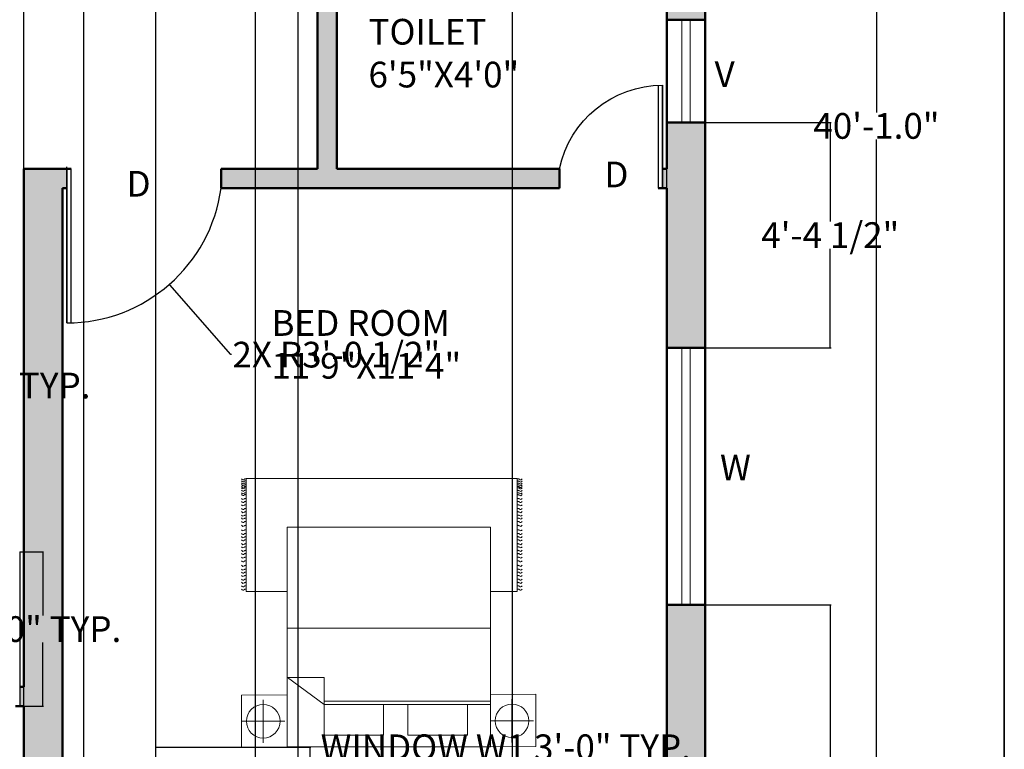
# Model space of a CAD drawing. Units: inches. Extents: x 125920 to 126336, y 366134 to 366735.
# Tile 3 of 6: x 126106 to 126336, y 366303 to 366473. Entities that reach past the tile are written whole.
import ezdxf

# ---------------------------------------------------------------- set-up
doc = ezdxf.new("R2010")
doc.units = ezdxf.units.IN
doc.header["$MEASUREMENT"] = 0
for name, color, linetype, lineweight in [('A-ANNO-DIMS', 2, 'Continuous', 18), ('A-ANNO-TEXT', 7, 'Continuous', 18), ('A-ANNO-TTLB', 7, 'Continuous', 35), ('A-AREA-IDEN', 7, 'Continuous', 25), ('A-DOOR', 3, 'Continuous', 25), ('A-FURN', 8, 'Continuous', 18), ('A-GLAZ', 4, 'Continuous', 18), ('A-WALL', 7, 'Continuous', 50)]:
    doc.layers.add(name, color=color, linetype=linetype, lineweight=lineweight)
doc.layers.add('A-WALL-PATT', color=18, linetype='Continuous', lineweight=13, true_color=0x000000)
doc.styles.get("Standard").update_dxf_attribs({"font": 'arial.ttf'})
doc.dimstyles.get("Standard").update_dxf_attribs({"dimtxt": 6, "dimasz": 0.18, "dimexe": 0.18, "dimexo": 0.0625, "dimgap": 0.09, "dimtad": 0, "dimtih": 1, "dimtoh": 1, "dimdec": 1, "dimzin": 0, "dimdsep": 46, "dimlunit": 3, "dimtxsty": 'Standard', "dimcen": 0.09, "dimadec": 0, "dimazin": 0, "dimtfac": 1, "dimtdec": 1, "dimtofl": 0, "dimtmove": 0, "dimatfit": 3, "dimfxl": 1, "dimtolj": 1, "dimtzin": 0, "dimarcsym": 0})

# ---------------------------------------------------------------- blocks, each defined once
blk = doc.blocks.new('*D4')
at = {"layer": 'A-ANNO-DIMS', "color": 0, "lineweight": -2, "transparency": 16777216}
for p, q in [((126266.54, 366688.79), (126306.57, 366688.79)), ((126306.39, 366688.61), (126306.39, 366451.45)), ((126306.39, 366207.97), (126306.39, 366445.14)), ((126266.54, 366207.79), (126306.57, 366207.79))]:
    blk.add_line(p, q, dxfattribs=at)
at = {"layer": 'A-ANNO-DIMS', "color": 0, "transparency": 16777216}
for points in [[(126306.36, 366688.61), (126306.42, 366688.61), (126306.39, 366688.79)], [(126306.36, 366207.97), (126306.42, 366207.97), (126306.39, 366207.79)]]:
    blk.add_solid(points, dxfattribs=at)
at = {"layer": 'Defpoints', "color": 0, "transparency": 16777216}
for p in [(126266.47, 366688.79), (126266.47, 366207.79), (126306.39, 366207.79)]:
    blk.add_point(p, dxfattribs=at)
at = {"layer": 'A-ANNO-DIMS', "color": 0, "transparency": 16777216, "insert": (126306.39, 366448.29), "char_height": 6, "attachment_point": 5}
blk.add_mtext('\\A1;40\'-1.0"', dxfattribs=at)
blk = doc.blocks.new('BED-DOUBLE-WITH-NIGHTSTANDS')
for p, q in [((5.6, 61.62), (5.6, 51.56)), ((63.65, 61.72), (63.65, 51.66)), ((10.63, 56.59), (0.57, 56.59)), ((68.68, 56.69), (58.62, 56.69)), ((49.39, 52.82), (10.63, 52.82)), ((49.44, 52), (10.63, 52)), ((49.39, 52.82), (58, 46.47)), ((49.44, 52.82), (49.44, 46.47)), ((49.44, 46.47), (58, 46.47)), ((58.05, 34.96), (10.63, 34.96)), ((4.36, 0), (4.36, 26.37)), ((4.36, 26.37), (10.65, 26.37)), ((58.05, 26.37), (67.59, 26.37)), ((67.59, 26.37), (67.59, 0)), ((67.59, 0), (4.36, 0))]:
    blk.add_line(p, q)
for points in [[(0, 50.39), (10.63, 50.5), (10.63, 62.68), (0, 62.58)], [(58.05, 62.68), (58.05, 11.37), (10.63, 11.37), (10.63, 62.68)], [(58.05, 50.5), (68.68, 50.6), (68.68, 62.78), (58.05, 62.68)], [(29.88, 59.98), (29.88, 52.82), (15.98, 52.82), (15.98, 59.98)], [(49.44, 59.98), (49.44, 52.82), (35.55, 52.82), (35.55, 59.98)]]:
    blk.add_lwpolyline(points, close=True)
for centre in [(5.6, 56.59), (63.65, 56.69)]:
    blk.add_circle(centre, 3.92)
for points, knots in [([(3.23, 25.84), (3.32, 25.96), (3.52, 26.2), (3.86, 25.96), (4.14, 25.78), (4.29, 25.89), (4.36, 25.94)], [0, 0, 0, 0, 0.400747, 0.791423, 1.067667, 1.29709, 1.29709, 1.29709, 1.29709]), ([(3.23, 25.06), (3.32, 25.18), (3.52, 25.42), (3.86, 25.18), (4.14, 25.01), (4.29, 25.11), (4.36, 25.16)], [0, 0, 0, 0, 0.400747, 0.791423, 1.067667, 1.29709, 1.29709, 1.29709, 1.29709]), ([(68.71, 25.84), (68.61, 25.96), (68.42, 26.2), (68.08, 25.96), (67.8, 25.78), (67.65, 25.89), (67.58, 25.94)], [0, 0, 0, 0, 0.400747, 0.791423, 1.067667, 1.29709, 1.29709, 1.29709, 1.29709]), ([(68.71, 25.06), (68.61, 25.18), (68.42, 25.42), (68.08, 25.18), (67.8, 25.01), (67.65, 25.11), (67.58, 25.16)], [0, 0, 0, 0, 0.400747, 0.791423, 1.067667, 1.29709, 1.29709, 1.29709, 1.29709]), ([(3.23, 24.24), (3.32, 24.36), (3.52, 24.6), (3.86, 24.36), (4.14, 24.19), (4.29, 24.3), (4.36, 24.34)], [0, 0, 0, 0, 0.400747, 0.791423, 1.067667, 1.29709, 1.29709, 1.29709, 1.29709]), ([(3.23, 23.51), (3.32, 23.63), (3.52, 23.87), (3.86, 23.63), (4.14, 23.46), (4.29, 23.57), (4.36, 23.62)], [0, 0, 0, 0, 0.400747, 0.791423, 1.067667, 1.29709, 1.29709, 1.29709, 1.29709]), ([(68.71, 24.24), (68.61, 24.36), (68.42, 24.6), (68.08, 24.36), (67.8, 24.19), (67.65, 24.3), (67.58, 24.34)], [0, 0, 0, 0, 0.400747, 0.791423, 1.067667, 1.29709, 1.29709, 1.29709, 1.29709]), ([(68.71, 23.51), (68.61, 23.63), (68.42, 23.87), (68.08, 23.63), (67.8, 23.46), (67.65, 23.57), (67.58, 23.62)], [0, 0, 0, 0, 0.400747, 0.791423, 1.067667, 1.29709, 1.29709, 1.29709, 1.29709]), ([(3.23, 22.63), (3.32, 22.75), (3.52, 22.99), (3.86, 22.75), (4.14, 22.58), (4.29, 22.69), (4.36, 22.73)], [0, 0, 0, 0, 0.400747, 0.791423, 1.067667, 1.29709, 1.29709, 1.29709, 1.29709]), ([(3.23, 21.88), (3.32, 22), (3.52, 22.24), (3.86, 22), (4.14, 21.83), (4.29, 21.93), (4.36, 21.98)], [0, 0, 0, 0, 0.400747, 0.791423, 1.067667, 1.29709, 1.29709, 1.29709, 1.29709]), ([(3.23, 21.15), (3.32, 21.27), (3.52, 21.51), (3.86, 21.27), (4.14, 21.1), (4.29, 21.21), (4.36, 21.25)], [0, 0, 0, 0, 0.400747, 0.791423, 1.067667, 1.29709, 1.29709, 1.29709, 1.29709]), ([(68.71, 22.63), (68.61, 22.75), (68.42, 22.99), (68.08, 22.75), (67.8, 22.58), (67.65, 22.69), (67.58, 22.73)], [0, 0, 0, 0, 0.400747, 0.791423, 1.067667, 1.29709, 1.29709, 1.29709, 1.29709]), ([(68.71, 21.88), (68.61, 22), (68.42, 22.24), (68.08, 22), (67.8, 21.83), (67.65, 21.93), (67.58, 21.98)], [0, 0, 0, 0, 0.400747, 0.791423, 1.067667, 1.29709, 1.29709, 1.29709, 1.29709]), ([(68.71, 21.15), (68.61, 21.27), (68.42, 21.51), (68.08, 21.27), (67.8, 21.1), (67.65, 21.21), (67.58, 21.25)], [0, 0, 0, 0, 0.400747, 0.791423, 1.067667, 1.29709, 1.29709, 1.29709, 1.29709]), ([(3.23, 20.27), (3.32, 20.39), (3.52, 20.63), (3.86, 20.39), (4.14, 20.22), (4.29, 20.32), (4.36, 20.37)], [0, 0, 0, 0, 0.400747, 0.791423, 1.067667, 1.29709, 1.29709, 1.29709, 1.29709]), ([(3.23, 19.23), (3.32, 19.35), (3.52, 19.59), (3.86, 19.35), (4.14, 19.18), (4.29, 19.29), (4.36, 19.33)], [0, 0, 0, 0, 0.400747, 0.791423, 1.067667, 1.29709, 1.29709, 1.29709, 1.29709]), ([(3.23, 18.35), (3.32, 18.47), (3.52, 18.71), (3.86, 18.47), (4.14, 18.3), (4.29, 18.4), (4.36, 18.45)], [0, 0, 0, 0, 0.400747, 0.791423, 1.067667, 1.29709, 1.29709, 1.29709, 1.29709]), ([(68.71, 20.27), (68.61, 20.39), (68.42, 20.63), (68.08, 20.39), (67.8, 20.22), (67.65, 20.32), (67.58, 20.37)], [0, 0, 0, 0, 0.400747, 0.791423, 1.067667, 1.29709, 1.29709, 1.29709, 1.29709]), ([(68.71, 19.23), (68.61, 19.35), (68.42, 19.59), (68.08, 19.35), (67.8, 19.18), (67.65, 19.29), (67.58, 19.33)], [0, 0, 0, 0, 0.400747, 0.791423, 1.067667, 1.29709, 1.29709, 1.29709, 1.29709]), ([(68.71, 18.35), (68.61, 18.47), (68.42, 18.71), (68.08, 18.47), (67.8, 18.3), (67.65, 18.4), (67.58, 18.45)], [0, 0, 0, 0, 0.400747, 0.791423, 1.067667, 1.29709, 1.29709, 1.29709, 1.29709]), ([(3.23, 17.53), (3.32, 17.65), (3.52, 17.89), (3.86, 17.65), (4.14, 17.48), (4.29, 17.59), (4.36, 17.64)], [0, 0, 0, 0, 0.400747, 0.791423, 1.067667, 1.29709, 1.29709, 1.29709, 1.29709]), ([(3.23, 16.76), (3.32, 16.88), (3.52, 17.12), (3.86, 16.88), (4.14, 16.7), (4.29, 16.81), (4.36, 16.86)], [0, 0, 0, 0, 0.400747, 0.791423, 1.067667, 1.29709, 1.29709, 1.29709, 1.29709]), ([(3.23, 15.94), (3.32, 16.06), (3.52, 16.3), (3.86, 16.06), (4.14, 15.89), (4.29, 16), (4.36, 16.04)], [0, 0, 0, 0, 0.400747, 0.791423, 1.067667, 1.29709, 1.29709, 1.29709, 1.29709]), ([(68.71, 17.53), (68.61, 17.65), (68.42, 17.89), (68.08, 17.65), (67.8, 17.48), (67.65, 17.59), (67.58, 17.64)], [0, 0, 0, 0, 0.400747, 0.791423, 1.067667, 1.29709, 1.29709, 1.29709, 1.29709]), ([(68.71, 16.76), (68.61, 16.88), (68.42, 17.12), (68.08, 16.88), (67.8, 16.7), (67.65, 16.81), (67.58, 16.86)], [0, 0, 0, 0, 0.400747, 0.791423, 1.067667, 1.29709, 1.29709, 1.29709, 1.29709]), ([(68.71, 15.94), (68.61, 16.06), (68.42, 16.3), (68.08, 16.06), (67.8, 15.89), (67.65, 16), (67.58, 16.04)], [0, 0, 0, 0, 0.400747, 0.791423, 1.067667, 1.29709, 1.29709, 1.29709, 1.29709]), ([(3.23, 15.21), (3.32, 15.33), (3.52, 15.57), (3.86, 15.33), (4.14, 15.16), (4.29, 15.27), (4.36, 15.32)], [0, 0, 0, 0, 0.400747, 0.791423, 1.067667, 1.29709, 1.29709, 1.29709, 1.29709]), ([(3.23, 14.33), (3.32, 14.45), (3.52, 14.69), (3.86, 14.45), (4.14, 14.28), (4.29, 14.38), (4.36, 14.43)], [0, 0, 0, 0, 0.400747, 0.791423, 1.067667, 1.29709, 1.29709, 1.29709, 1.29709]), ([(3.23, 13.58), (3.32, 13.7), (3.52, 13.94), (3.86, 13.7), (4.14, 13.53), (4.29, 13.63), (4.36, 13.68)], [0, 0, 0, 0, 0.400747, 0.791423, 1.067667, 1.29709, 1.29709, 1.29709, 1.29709]), ([(68.71, 15.21), (68.61, 15.33), (68.42, 15.57), (68.08, 15.33), (67.8, 15.16), (67.65, 15.27), (67.58, 15.32)], [0, 0, 0, 0, 0.400747, 0.791423, 1.067667, 1.29709, 1.29709, 1.29709, 1.29709]), ([(68.71, 14.33), (68.61, 14.45), (68.42, 14.69), (68.08, 14.45), (67.8, 14.28), (67.65, 14.38), (67.58, 14.43)], [0, 0, 0, 0, 0.400747, 0.791423, 1.067667, 1.29709, 1.29709, 1.29709, 1.29709]), ([(68.71, 13.58), (68.61, 13.7), (68.42, 13.94), (68.08, 13.7), (67.8, 13.53), (67.65, 13.63), (67.58, 13.68)], [0, 0, 0, 0, 0.400747, 0.791423, 1.067667, 1.29709, 1.29709, 1.29709, 1.29709]), ([(3.23, 12.85), (3.32, 12.97), (3.52, 13.21), (3.86, 12.97), (4.14, 12.8), (4.29, 12.9), (4.36, 12.95)], [0, 0, 0, 0, 0.400747, 0.791423, 1.067667, 1.29709, 1.29709, 1.29709, 1.29709]), ([(3.23, 11.97), (3.32, 12.09), (3.52, 12.33), (3.86, 12.09), (4.14, 11.92), (4.29, 12.02), (4.36, 12.07)], [0, 0, 0, 0, 0.400747, 0.791423, 1.067667, 1.29709, 1.29709, 1.29709, 1.29709]), ([(68.71, 12.85), (68.61, 12.97), (68.42, 13.21), (68.08, 12.97), (67.8, 12.8), (67.65, 12.9), (67.58, 12.95)], [0, 0, 0, 0, 0.400747, 0.791423, 1.067667, 1.29709, 1.29709, 1.29709, 1.29709]), ([(68.71, 11.97), (68.61, 12.09), (68.42, 12.33), (68.08, 12.09), (67.8, 11.92), (67.65, 12.02), (67.58, 12.07)], [0, 0, 0, 0, 0.400747, 0.791423, 1.067667, 1.29709, 1.29709, 1.29709, 1.29709]), ([(3.23, 10.93), (3.32, 11.05), (3.52, 11.29), (3.86, 11.05), (4.14, 10.88), (4.29, 10.99), (4.36, 11.03)], [0, 0, 0, 0, 0.400747, 0.791423, 1.067667, 1.29709, 1.29709, 1.29709, 1.29709]), ([(3.23, 10.05), (3.32, 10.17), (3.52, 10.41), (3.86, 10.17), (4.14, 10), (4.29, 10.1), (4.36, 10.15)], [0, 0, 0, 0, 0.400747, 0.791423, 1.067667, 1.29709, 1.29709, 1.29709, 1.29709]), ([(3.23, 9.23), (3.32, 9.35), (3.52, 9.59), (3.86, 9.35), (4.14, 9.18), (4.29, 9.29), (4.36, 9.34)], [0, 0, 0, 0, 0.400747, 0.791423, 1.067667, 1.29709, 1.29709, 1.29709, 1.29709]), ([(68.71, 10.93), (68.61, 11.05), (68.42, 11.29), (68.08, 11.05), (67.8, 10.88), (67.65, 10.99), (67.58, 11.03)], [0, 0, 0, 0, 0.400747, 0.791423, 1.067667, 1.29709, 1.29709, 1.29709, 1.29709]), ([(68.71, 10.05), (68.61, 10.17), (68.42, 10.41), (68.08, 10.17), (67.8, 10), (67.65, 10.1), (67.58, 10.15)], [0, 0, 0, 0, 0.400747, 0.791423, 1.067667, 1.29709, 1.29709, 1.29709, 1.29709]), ([(68.71, 9.23), (68.61, 9.35), (68.42, 9.59), (68.08, 9.35), (67.8, 9.18), (67.65, 9.29), (67.58, 9.34)], [0, 0, 0, 0, 0.400747, 0.791423, 1.067667, 1.29709, 1.29709, 1.29709, 1.29709]), ([(3.23, 8.54), (3.32, 8.66), (3.52, 8.9), (3.86, 8.66), (4.14, 8.49), (4.29, 8.6), (4.36, 8.65)], [0, 0, 0, 0, 0.400747, 0.791423, 1.067667, 1.29709, 1.29709, 1.29709, 1.29709]), ([(3.23, 7.73), (3.32, 7.85), (3.52, 8.09), (3.86, 7.85), (4.14, 7.68), (4.29, 7.78), (4.36, 7.83)], [0, 0, 0, 0, 0.400747, 0.791423, 1.067667, 1.29709, 1.29709, 1.29709, 1.29709]), ([(3.23, 7), (3.32, 7.12), (3.52, 7.36), (3.86, 7.12), (4.14, 6.95), (4.29, 7.05), (4.36, 7.1)], [0, 0, 0, 0, 0.400747, 0.791423, 1.067667, 1.29709, 1.29709, 1.29709, 1.29709]), ([(68.71, 8.54), (68.61, 8.66), (68.42, 8.9), (68.08, 8.66), (67.8, 8.49), (67.65, 8.6), (67.58, 8.65)], [0, 0, 0, 0, 0.400747, 0.791423, 1.067667, 1.29709, 1.29709, 1.29709, 1.29709]), ([(68.71, 7.73), (68.61, 7.85), (68.42, 8.09), (68.08, 7.85), (67.8, 7.68), (67.65, 7.78), (67.58, 7.83)], [0, 0, 0, 0, 0.400747, 0.791423, 1.067667, 1.29709, 1.29709, 1.29709, 1.29709]), ([(68.71, 7), (68.61, 7.12), (68.42, 7.36), (68.08, 7.12), (67.8, 6.95), (67.65, 7.05), (67.58, 7.1)], [0, 0, 0, 0, 0.400747, 0.791423, 1.067667, 1.29709, 1.29709, 1.29709, 1.29709]), ([(3.23, 6.12), (3.32, 6.24), (3.52, 6.48), (3.86, 6.24), (4.14, 6.07), (4.29, 6.17), (4.36, 6.22)], [0, 0, 0, 0, 0.400747, 0.791423, 1.067667, 1.29709, 1.29709, 1.29709, 1.29709]), ([(3.23, 5.36), (3.32, 5.49), (3.52, 5.73), (3.86, 5.49), (4.14, 5.31), (4.29, 5.42), (4.36, 5.47)], [0, 0, 0, 0, 0.400747, 0.791423, 1.067667, 1.29709, 1.29709, 1.29709, 1.29709]), ([(3.23, 4.64), (3.32, 4.76), (3.52, 5), (3.86, 4.76), (4.14, 4.59), (4.29, 4.69), (4.36, 4.74)], [0, 0, 0, 0, 0.400747, 0.791423, 1.067667, 1.29709, 1.29709, 1.29709, 1.29709]), ([(68.71, 6.12), (68.61, 6.24), (68.42, 6.48), (68.08, 6.24), (67.8, 6.07), (67.65, 6.17), (67.58, 6.22)], [0, 0, 0, 0, 0.400747, 0.791423, 1.067667, 1.29709, 1.29709, 1.29709, 1.29709]), ([(68.71, 5.36), (68.61, 5.49), (68.42, 5.73), (68.08, 5.49), (67.8, 5.31), (67.65, 5.42), (67.58, 5.47)], [0, 0, 0, 0, 0.400747, 0.791423, 1.067667, 1.29709, 1.29709, 1.29709, 1.29709]), ([(68.71, 4.64), (68.61, 4.76), (68.42, 5), (68.08, 4.76), (67.8, 4.59), (67.66, 4.69), (67.59, 4.73)], [0, 0, 0, 0, 0.400747, 0.791423, 1.067667, 1.283686, 1.283686, 1.283686, 1.283686]), ([(3.23, 3.75), (3.32, 3.88), (3.52, 4.12), (3.86, 3.88), (4.14, 3.7), (4.29, 3.81), (4.36, 3.86)], [0, 0, 0, 0, 0.400747, 0.791423, 1.067667, 1.29709, 1.29709, 1.29709, 1.29709]), ([(3.23, 3.33), (3.32, 3.45), (3.52, 3.7), (3.86, 3.44), (4.14, 3.27), (4.29, 3.38), (4.36, 3.43)], [0, 0, 0, 0, 0.407265, 0.802015, 1.07826, 1.307683, 1.307683, 1.307683, 1.307683]), ([(3.23, 2.76), (3.32, 2.88), (3.52, 3.12), (3.86, 2.88), (4.14, 2.71), (4.29, 2.81), (4.36, 2.86)], [0, 0, 0, 0, 0.400747, 0.791423, 1.067667, 1.29709, 1.29709, 1.29709, 1.29709]), ([(3.23, 2.18), (3.32, 2.31), (3.52, 2.55), (3.86, 2.31), (4.14, 2.13), (4.29, 2.24), (4.36, 2.29)], [0, 0, 0, 0, 0.400747, 0.791423, 1.067667, 1.29709, 1.29709, 1.29709, 1.29709]), ([(68.71, 3.75), (68.61, 3.88), (68.42, 4.11), (68.08, 3.88), (67.8, 3.7), (67.66, 3.81), (67.59, 3.85)], [0, 0, 0, 0, 0.400747, 0.791423, 1.067667, 1.283686, 1.283686, 1.283686, 1.283686]), ([(68.71, 3.33), (68.61, 3.45), (68.42, 3.69), (68.08, 3.45), (67.8, 3.27), (67.66, 3.38), (67.59, 3.42)], [0, 0, 0, 0, 0.402903, 0.794912, 1.071156, 1.287177, 1.287177, 1.287177, 1.287177]), ([(68.71, 2.73), (68.61, 2.85), (68.42, 3.09), (68.08, 2.85), (67.8, 2.68), (67.66, 2.78), (67.59, 2.82)], [0, 0, 0, 0, 0.400747, 0.791423, 1.067667, 1.283686, 1.283686, 1.283686, 1.283686]), ([(68.71, 2.16), (68.61, 2.28), (68.42, 2.52), (68.08, 2.28), (67.8, 2.11), (67.66, 2.21), (67.59, 2.25)], [0, 0, 0, 0, 0.400747, 0.791423, 1.067667, 1.283686, 1.283686, 1.283686, 1.283686]), ([(3.23, 1.88), (3.32, 2), (3.52, 2.24), (3.86, 2), (4.14, 1.82), (4.29, 1.93), (4.36, 1.98)], [0, 0, 0, 0, 0.400747, 0.791423, 1.067667, 1.29709, 1.29709, 1.29709, 1.29709]), ([(3.23, 1.46), (3.32, 1.58), (3.52, 1.82), (3.86, 1.58), (4.14, 1.41), (4.29, 1.51), (4.36, 1.56)], [0, 0, 0, 0, 0.400747, 0.791423, 1.067667, 1.29709, 1.29709, 1.29709, 1.29709]), ([(3.23, 1.06), (3.32, 1.18), (3.52, 1.42), (3.86, 1.18), (4.14, 1.01), (4.29, 1.11), (4.36, 1.16)], [0, 0, 0, 0, 0.400747, 0.791423, 1.067667, 1.29709, 1.29709, 1.29709, 1.29709]), ([(3.23, 0.57), (3.32, 0.7), (3.52, 0.94), (3.86, 0.7), (4.14, 0.52), (4.29, 0.63), (4.36, 0.68)], [0, 0, 0, 0, 0.400747, 0.791423, 1.067667, 1.29709, 1.29709, 1.29709, 1.29709]), ([(3.23, 0.07), (3.32, 0.19), (3.52, 0.43), (3.86, 0.19), (4.14, 0.02), (4.29, 0.13), (4.36, 0.18)], [0, 0, 0, 0, 0.400747, 0.791423, 1.067667, 1.29709, 1.29709, 1.29709, 1.29709]), ([(68.71, 1.43), (68.61, 1.55), (68.42, 1.79), (68.08, 1.55), (67.8, 1.38), (67.65, 1.48), (67.58, 1.53)], [0, 0, 0, 0, 0.400747, 0.791423, 1.067667, 1.29709, 1.29709, 1.29709, 1.29709]), ([(68.71, 1.03), (68.61, 1.15), (68.42, 1.39), (68.08, 1.15), (67.8, 0.98), (67.65, 1.09), (67.58, 1.13)], [0, 0, 0, 0, 0.400747, 0.791423, 1.067667, 1.29709, 1.29709, 1.29709, 1.29709]), ([(68.71, 0.55), (68.61, 0.67), (68.42, 0.91), (68.08, 0.67), (67.8, 0.49), (67.65, 0.6), (67.58, 0.65)], [0, 0, 0, 0, 0.400747, 0.791423, 1.067667, 1.29709, 1.29709, 1.29709, 1.29709]), ([(68.71, 0.07), (68.61, 0.19), (68.42, 0.43), (68.08, 0.19), (67.8, 0.02), (67.65, 0.13), (67.58, 0.18)], [0, 0, 0, 0, 0.400747, 0.791423, 1.067667, 1.29709, 1.29709, 1.29709, 1.29709]), ([(68.71, 1.85), (68.61, 1.97), (68.42, 2.21), (68.08, 1.97), (67.8, 1.8), (67.66, 1.9), (67.59, 1.94)], [0, 0, 0, 0, 0.400747, 0.791423, 1.067667, 1.283686, 1.283686, 1.283686, 1.283686])]:
    blk.add_open_spline(points, degree=3, knots=knots)
blk = doc.blocks.new('WIN-60')
for p, q in [((0, 0), (0, 60)), ((3.5, 0), (3.5, 60)), ((5.5, 60), (5.5, 0)), ((9, 60), (9, 0))]:
    blk.add_line(p, q)
blk = doc.blocks.new('VENT-24')
for p, q in [((0, 0), (0, 24)), ((3.5, 0), (3.5, 24)), ((5.5, 24), (5.5, 0)), ((9, 24), (9, 0))]:
    blk.add_line(p, q)
blk = doc.blocks.new('DOOR-36-WALL-4_5')
for p, q in [((0, 36), (0, 0)), ((0, 36), (1, 36)), ((1, 0), (1, 36))]:
    blk.add_line(p, q)
blk.add_arc((0, 36.32), 36.32, 270, 352.3719)
blk = doc.blocks.new('DOOR-24-WALL-4_5')
for p, q in [((0, 1), (24, 1)), ((24, 0), (24, 1)), ((24, 0), (0, 0))]:
    blk.add_line(p, q)
blk.add_arc((24.52, 0), 24.52, 101.8123, 180)
blk = doc.blocks.new('*D15')
at = {"layer": 'A-ANNO-DIMS', "color": 0, "lineweight": -2, "transparency": 16777216}
for p, q in [((126138.23, 366297.86), (126138.23, 366303.37)), ((126138.41, 366303.19), (126174.05, 366303.19)), ((126174.23, 366297.86), (126174.23, 366303.37)), ((126174.23, 366303.19), (126174.41, 366303.19))]:
    blk.add_line(p, q, dxfattribs=at)
at = {"layer": 'A-ANNO-DIMS', "color": 0, "transparency": 16777216}
for points in [[(126138.41, 366303.22), (126138.41, 366303.16), (126138.23, 366303.19)], [(126174.05, 366303.22), (126174.05, 366303.16), (126174.23, 366303.19)]]:
    blk.add_solid(points, dxfattribs=at)
at = {"layer": 'Defpoints', "color": 0, "transparency": 16777216}
for p in [(126174.23, 366303.19), (126138.23, 366297.79), (126174.23, 366297.79)]:
    blk.add_point(p, dxfattribs=at)
at = {"layer": 'A-ANNO-DIMS', "color": 0, "transparency": 16777216, "insert": (126219.91, 366303.19), "char_height": 6, "attachment_point": 5}
blk.add_mtext('\\A1;WINDOW W1 3\'-0" TYP.', dxfattribs=at)
blk = doc.blocks.new('*D21')
at = {"layer": 'A-ANNO-DIMS', "color": 0, "lineweight": -2, "transparency": 16777216}
for p, q in [((126007.38, 366379.47), (126007.38, 366387.84)), ((126007.56, 366387.66), (126062.24, 366387.66)), ((126062.42, 366379.47), (126062.42, 366387.84)), ((126062.42, 366387.66), (126062.6, 366387.66))]:
    blk.add_line(p, q, dxfattribs=at)
at = {"layer": 'A-ANNO-DIMS', "color": 0, "transparency": 16777216}
for points in [[(126007.56, 366387.69), (126007.56, 366387.63), (126007.38, 366387.66)], [(126062.24, 366387.69), (126062.24, 366387.63), (126062.42, 366387.66)]]:
    blk.add_solid(points, dxfattribs=at)
at = {"layer": 'Defpoints', "color": 0, "transparency": 16777216}
for p in [(126062.42, 366387.66), (126007.38, 366379.4), (126062.42, 366379.4)]:
    blk.add_point(p, dxfattribs=at)
at = {"layer": 'A-ANNO-DIMS', "color": 0, "transparency": 16777216, "insert": (126093.54, 366387.66), "char_height": 6, "attachment_point": 5}
blk.add_mtext('\\A1;SOFA 4\'-7" TYP.', dxfattribs=at)
blk = doc.blocks.new('*D24')
at = {"layer": 'A-ANNO-DIMS', "color": 0, "lineweight": -2, "transparency": 16777216}
for p, q in [((126106.54, 366348.79), (126112.05, 366348.79)), ((126111.87, 366348.61), (126111.87, 366333.95)), ((126111.87, 366312.97), (126111.87, 366327.64)), ((126106.54, 366312.79), (126112.05, 366312.79))]:
    blk.add_line(p, q, dxfattribs=at)
at = {"layer": 'A-ANNO-DIMS', "color": 0, "transparency": 16777216}
for points in [[(126111.84, 366348.61), (126111.9, 366348.61), (126111.87, 366348.79)], [(126111.84, 366312.97), (126111.9, 366312.97), (126111.87, 366312.79)]]:
    blk.add_solid(points, dxfattribs=at)
at = {"layer": 'Defpoints', "color": 0, "transparency": 16777216}
for p in [(126106.47, 366348.79), (126106.47, 366312.79), (126111.87, 366312.79)]:
    blk.add_point(p, dxfattribs=at)
at = {"layer": 'A-ANNO-DIMS', "color": 0, "transparency": 16777216, "insert": (126111.87, 366330.79), "char_height": 6, "attachment_point": 5}
blk.add_mtext('\\A1;3\'-0" TYP.', dxfattribs=at)
blk = doc.blocks.new('*D32')
at = {"layer": 'A-ANNO-DIMS', "color": 0, "lineweight": -2, "transparency": 16777216}
for p, q in [((126266.54, 366336.48), (126295.8, 366336.48)), ((126295.62, 366336.3), (126295.62, 366275.33)), ((126295.62, 366207.97), (126295.62, 366268.94)), ((126266.54, 366207.79), (126295.8, 366207.79))]:
    blk.add_line(p, q, dxfattribs=at)
at = {"layer": 'A-ANNO-DIMS', "color": 0, "transparency": 16777216}
for points in [[(126295.59, 366336.3), (126295.65, 366336.3), (126295.62, 366336.48)], [(126295.59, 366207.97), (126295.65, 366207.97), (126295.62, 366207.79)]]:
    blk.add_solid(points, dxfattribs=at)
at = {"layer": 'Defpoints', "color": 0, "transparency": 16777216}
for p in [(126266.47, 366336.48), (126295.62, 366336.48), (126266.47, 366207.79)]:
    blk.add_point(p, dxfattribs=at)
at = {"layer": 'A-ANNO-DIMS', "color": 0, "transparency": 16777216, "insert": (126295.62, 366272.14), "char_height": 6, "attachment_point": 5}
blk.add_mtext('\\A1;10\'-8 1/2"', dxfattribs=at)
blk = doc.blocks.new('*D33')
at = {"layer": 'A-ANNO-DIMS', "color": 0, "lineweight": -2, "transparency": 16777216}
for p, q in [((126266.54, 366449.1), (126295.8, 366449.1)), ((126295.62, 366448.92), (126295.62, 366425.98)), ((126295.62, 366396.66), (126295.62, 366419.6)), ((126266.54, 366396.48), (126295.8, 366396.48))]:
    blk.add_line(p, q, dxfattribs=at)
at = {"layer": 'A-ANNO-DIMS', "color": 0, "transparency": 16777216}
for points in [[(126295.59, 366448.92), (126295.65, 366448.92), (126295.62, 366449.1)], [(126295.59, 366396.66), (126295.65, 366396.66), (126295.62, 366396.48)]]:
    blk.add_solid(points, dxfattribs=at)
at = {"layer": 'Defpoints', "color": 0, "transparency": 16777216}
for p in [(126266.47, 366449.1), (126295.62, 366449.1), (126266.47, 366396.48)]:
    blk.add_point(p, dxfattribs=at)
at = {"layer": 'A-ANNO-DIMS', "color": 0, "transparency": 16777216, "insert": (126295.62, 366422.79), "char_height": 6, "attachment_point": 5}
blk.add_mtext('\\A1;4\'-4 1/2"', dxfattribs=at)
blk = doc.blocks.new('*D40')
at = {"layer": 'A-ANNO-DIMS', "color": 0, "lineweight": -2, "transparency": 16777216}
for p, q in [((126107.47, 366288.86), (126107.47, 366718.12)), ((126107.65, 366717.94), (126114.73, 366717.94)), ((126138.05, 366717.94), (126130.97, 366717.94)), ((126138.23, 366288.86), (126138.23, 366718.12))]:
    blk.add_line(p, q, dxfattribs=at)
at = {"layer": 'A-ANNO-DIMS', "color": 0, "transparency": 16777216}
for points in [[(126107.65, 366717.97), (126107.65, 366717.91), (126107.47, 366717.94)], [(126138.05, 366717.97), (126138.05, 366717.91), (126138.23, 366717.94)]]:
    blk.add_solid(points, dxfattribs=at)
at = {"layer": 'Defpoints', "color": 0, "transparency": 16777216}
for p in [(126138.23, 366717.94), (126107.47, 366288.79), (126138.23, 366288.79)]:
    blk.add_point(p, dxfattribs=at)
at = {"layer": 'A-ANNO-DIMS', "color": 0, "transparency": 16777216, "insert": (126122.85, 366717.94), "char_height": 6, "attachment_point": 5}
blk.add_mtext('\\A1;2\'-7"', dxfattribs=at)
blk = doc.blocks.new('*D41')
at = {"layer": 'A-ANNO-DIMS', "color": 0, "lineweight": -2, "transparency": 16777216}
for p, q in [((126121.47, 366216.86), (126121.47, 366718.12)), ((126121.65, 366717.94), (126163.4, 366717.94)), ((126221.29, 366717.94), (126179.54, 366717.94)), ((126221.47, 366216.86), (126221.47, 366718.12))]:
    blk.add_line(p, q, dxfattribs=at)
at = {"layer": 'A-ANNO-DIMS', "color": 0, "transparency": 16777216}
for points in [[(126121.65, 366717.97), (126121.65, 366717.91), (126121.47, 366717.94)], [(126221.29, 366717.97), (126221.29, 366717.91), (126221.47, 366717.94)]]:
    blk.add_solid(points, dxfattribs=at)
at = {"layer": 'Defpoints', "color": 0, "transparency": 16777216}
for p in [(126221.47, 366717.94), (126121.47, 366216.79), (126221.47, 366216.79)]:
    blk.add_point(p, dxfattribs=at)
at = {"layer": 'A-ANNO-DIMS', "color": 0, "transparency": 16777216, "insert": (126171.47, 366717.94), "char_height": 6, "attachment_point": 5}
blk.add_mtext('\\A1;8\'-4"', dxfattribs=at)
blk = doc.blocks.new('*D43')
at = {"layer": 'A-ANNO-DIMS', "color": 0, "lineweight": -2, "transparency": 16777216}
for p, q in [((126221.47, 366216.86), (126221.47, 366718.12)), ((126221.65, 366717.94), (126231.41, 366717.94)), ((126257.29, 366717.94), (126247.54, 366717.94)), ((126257.47, 366216.86), (126257.47, 366718.12))]:
    blk.add_line(p, q, dxfattribs=at)
at = {"layer": 'A-ANNO-DIMS', "color": 0, "transparency": 16777216}
for points in [[(126221.65, 366717.97), (126221.65, 366717.91), (126221.47, 366717.94)], [(126257.29, 366717.97), (126257.29, 366717.91), (126257.47, 366717.94)]]:
    blk.add_solid(points, dxfattribs=at)
at = {"layer": 'Defpoints', "color": 0, "transparency": 16777216}
for p in [(126257.47, 366717.94), (126221.47, 366216.79), (126257.47, 366216.79)]:
    blk.add_point(p, dxfattribs=at)
at = {"layer": 'A-ANNO-DIMS', "color": 0, "transparency": 16777216, "insert": (126239.47, 366717.94), "char_height": 6, "attachment_point": 5}
blk.add_mtext('\\A1;3\'-0"', dxfattribs=at)
blk = doc.blocks.new('*D44')
at = {"layer": 'A-ANNO-DIMS', "color": 0, "lineweight": -2, "transparency": 16777216}
for p, q in [((126161.47, 366252.86), (126161.47, 366718.12)), ((126161.65, 366717.94), (126171.29, 366717.94)), ((126171.47, 366252.86), (126171.47, 366718.12)), ((126171.47, 366717.94), (126171.65, 366717.94))]:
    blk.add_line(p, q, dxfattribs=at)
at = {"layer": 'A-ANNO-DIMS', "color": 0, "transparency": 16777216}
for points in [[(126161.65, 366717.97), (126161.65, 366717.91), (126161.47, 366717.94)], [(126171.29, 366717.97), (126171.29, 366717.91), (126171.47, 366717.94)]]:
    blk.add_solid(points, dxfattribs=at)
at = {"layer": 'Defpoints', "color": 0, "transparency": 16777216}
for p in [(126171.47, 366717.94), (126161.47, 366252.79), (126171.47, 366252.79)]:
    blk.add_point(p, dxfattribs=at)
at = {"layer": 'A-ANNO-DIMS', "color": 0, "transparency": 16777216, "insert": (126182.05, 366717.94), "char_height": 6, "attachment_point": 5}
blk.add_mtext('\\A1;0\'-10"', dxfattribs=at)
blk = doc.blocks.new('*D49')
at = {"layer": 'A-ANNO-DIMS', "color": 0, "lineweight": -2, "transparency": 16777216}
for p, q in [((126117.38, 366438.62), (126117.56, 366438.62)), ((126117.47, 366438.53), (126117.47, 366438.71)), ((126155.74, 366394.88), (126141.51, 366411.15)), ((126155.92, 366394.88), (126155.74, 366394.88))]:
    blk.add_line(p, q, dxfattribs=at)
at = {"layer": 'A-ANNO-DIMS', "color": 0, "transparency": 16777216}
blk.add_solid([(126141.53, 366411.17), (126141.49, 366411.13), (126141.39, 366411.28)], dxfattribs=at)
at = {"layer": 'Defpoints', "color": 0, "transparency": 16777216}
for p in [(126117.47, 366438.62), (126141.39, 366411.28)]:
    blk.add_point(p, dxfattribs=at)
at = {"layer": 'A-ANNO-DIMS', "color": 0, "transparency": 16777216, "insert": (126180.35, 366394.88), "char_height": 6, "attachment_point": 5}
blk.add_mtext('\\A1;2X R3\'-0 1/2"', dxfattribs=at)

msp = doc.modelspace()

# ---------------------------------------------------------------- hatches: boundary and pattern name
at = {"layer": 'A-WALL-PATT'}
h = msp.add_hatch(color=256, dxfattribs=at)
h.dxf.hatch_style = 1
h.paths.add_polyline_path([(126266.47, 366688.79), (125966.47, 366688.79), (125966.47, 366649.55), (125975.47, 366649.55), (125975.47, 366679.79), (126107.47, 366679.79), (126107.47, 366547.79), (126106.47, 366547.79), (126106.47, 366538.79), (126107.47, 366538.79), (126117.47, 366538.79), (126117.47, 366547.79), (126116.47, 366547.79), (126116.47, 366679.79), (126257.47, 366679.79), (126257.47, 366648.33), (126266.47, 366648.33)])
h.paths.add_polyline_path([(126070.47, 366547.79), (125975.47, 366547.79), (125975.47, 366589.55), (125966.47, 366589.55), (125966.47, 366528.42), (125975.47, 366528.42), (125975.47, 366538.79), (126059.47, 366538.79), (126059.47, 366515.79), (126063.97, 366515.79), (126063.97, 366538.79), (126070.47, 366538.79)])
h.paths.add_polyline_path([(125975.47, 366486.29), (126063.97, 366486.29), (126063.97, 366491.79), (126059.47, 366491.79), (126059.47, 366490.79), (125975.47, 366490.79), (125975.47, 366504.42), (125966.47, 366504.42), (125966.47, 366437.07), (125975.47, 366437.07)])
h.paths.add_polyline_path([(125975.47, 366312.79), (126022.47, 366312.79), (126022.47, 366317.29), (125975.47, 366317.29), (125975.47, 366377.07), (125966.47, 366377.07), (125966.47, 366207.79), (125987.64, 366207.79), (125987.64, 366216.79), (125975.47, 366216.79)])
h.paths.add_polyline_path([(126063.97, 366216.79), (126063.97, 366312.79), (126070.47, 366312.79), (126070.47, 366317.29), (126058.47, 366317.29), (126058.47, 366312.79), (126059.47, 366312.79), (126059.47, 366216.79), (126047.64, 366216.79), (126047.64, 366207.79), (126063.97, 366207.79)])
h.paths.add_polyline_path([(126221.47, 366216.79), (126116.47, 366216.79), (126107.47, 366216.79), (126107.47, 366207.79), (126221.47, 366207.79)])
h.paths.add_polyline_path([(126266.47, 366336.48), (126257.47, 366336.48), (126257.47, 366297.79), (126174.23, 366297.79), (126174.23, 366288.79), (126257.47, 366288.79), (126257.47, 366207.79), (126266.47, 366207.79)])
h.paths.add_polyline_path([(126138.23, 366297.79), (126116.47, 366297.79), (126116.47, 366433.79), (126117.47, 366433.79), (126117.47, 366438.29), (126116.47, 366438.29), (126107.47, 366438.29), (126107.47, 366317.29), (126106.47, 366317.29), (126106.47, 366312.79), (126107.47, 366312.79), (126107.47, 366288.79), (126116.47, 366288.79), (126138.23, 366288.79)])
h.paths.add_polyline_path([(126266.47, 366449.1), (126257.47, 366449.1), (126257.47, 366438.29), (126256.47, 366438.29), (126256.47, 366433.79), (126257.47, 366433.79), (126257.47, 366396.48), (126266.47, 366396.48)])
h.paths.add_polyline_path([(126232.47, 366438.29), (126180.47, 366438.29), (126180.47, 366486.29), (126257.47, 366486.29), (126257.47, 366473.1), (126266.47, 366473.1), (126266.47, 366504.78), (126257.47, 366504.78), (126257.47, 366490.79), (126180.47, 366490.79), (126180.47, 366538.79), (126232.47, 366538.79), (126232.47, 366547.79), (126153.47, 366547.79), (126153.47, 366538.79), (126175.97, 366538.79), (126175.97, 366438.29), (126153.47, 366438.29), (126153.47, 366433.79), (126232.47, 366433.79)])
h.paths.add_polyline_path([(126266.47, 366588.33), (126257.47, 366588.33), (126257.47, 366547.79), (126256.47, 366547.79), (126256.47, 366538.79), (126257.47, 366538.79), (126257.47, 366528.78), (126266.47, 366528.78)])

# ---------------------------------------------------------------- linework, layer by layer
at = {"layer": 'A-ANNO-TTLB'}
msp.add_lwpolyline([(125932.73, 366735.48), (126336.24, 366735.48), (126336.24, 366133.52), (125932.73, 366133.52)], close=True, dxfattribs=at)
at = {"layer": 'A-DOOR'}
for p, q in [((126256.47, 366457.79), (126256.47, 366433.79)), ((126116.47, 366438.29), (126117.47, 366438.29)), ((126117.47, 366402.29), (126117.47, 366438.29)), ((126257.47, 366433.79), (126256.47, 366433.79)), ((126106.47, 366348.79), (126106.47, 366312.79)), ((126107.47, 366312.79), (126106.47, 366312.79))]:
    msp.add_line(p, q, dxfattribs=at)
at = {"layer": 'A-WALL'}
for p, q in [((126266.47, 366688.79), (126266.47, 366207.79)), ((126175.97, 366538.79), (126175.97, 366438.29)), ((126180.47, 366486.29), (126180.47, 366438.29)), ((126257.47, 366486.29), (126257.47, 366438.29)), ((126257.47, 366473.1), (126266.47, 366473.1)), ((126266.47, 366449.1), (126257.47, 366449.1)), ((126107.47, 366438.29), (126107.47, 366317.29)), ((126107.47, 366438.29), (126118.47, 366438.29)), ((126153.47, 366438.29), (126153.47, 366433.79)), ((126153.47, 366438.29), (126175.97, 366438.29)), ((126180.47, 366438.29), (126232.47, 366438.29)), ((126232.47, 366433.79), (126232.47, 366438.29)), ((126256.47, 366438.29), (126257.47, 366438.29)), ((126116.47, 366433.79), (126116.47, 366297.79)), ((126116.47, 366433.79), (126117.47, 366433.79)), ((126153.47, 366433.79), (126232.47, 366433.79)), ((126255.47, 366433.79), (126257.47, 366433.79)), ((126257.47, 366433.79), (126257.47, 366297.79)), ((126257.47, 366396.48), (126266.47, 366396.48)), ((126266.47, 366336.48), (126257.47, 366336.48)), ((126106.47, 366317.29), (126107.47, 366317.29)), ((126105.47, 366312.79), (126107.47, 366312.79)), ((126107.47, 366312.79), (126107.47, 366288.79))]:
    msp.add_line(p, q, dxfattribs=at)

# ---------------------------------------------------------------- block references
at = {"layer": 'A-DOOR', "extrusion": (0, 0, -1), "zscale": -1, "rotation": 269.9999999998154}
msp.add_blockref('DOOR-24-WALL-4_5', (-126256.47, 366457.79), dxfattribs=at)
at = {"layer": 'A-DOOR'}
msp.add_blockref('DOOR-36-WALL-4_5', (126117.47, 366402.29), dxfattribs=at)
at = {"layer": 'A-FURN', "rotation": 180}
msp.add_blockref('BED-DOUBLE-WITH-NIGHTSTANDS', (126226.95, 366365.96), dxfattribs=at)
at = {"layer": 'A-GLAZ'}
for name, p in [('VENT-24', (126257.47, 366449.1)), ('WIN-60', (126257.47, 366336.48))]:
    msp.add_blockref(name, p, dxfattribs=at)

# ---------------------------------------------------------------- texts
at = {"layer": 'A-ANNO-TEXT', "char_height": 6, "attachment_point": 1}
for s, width, insert in [('V', 9.8961, (126268.62, 366463.4)), ('D', 9.6923, (126242.9, 366439.95)), ('D', 9.6923, (126131.4, 366437.78)), ('W', 14.507, (126269.9, 366371.5))]:
    msp.add_mtext_dynamic_manual_height_columns(s, width=width, gutter_width=30, heights=[0], dxfattribs=dict(at, insert=insert))
at = {"layer": 'A-AREA-IDEN', "char_height": 6, "attachment_point": 1}
for s, width, insert in [('TOILET\\P6\'5"X4\'0"', 40.1985, (126187.86, 366473.28)), ('BED ROOM\\P11\'9"X11\'4"', 61.589, (126165.23, 366405.27))]:
    msp.add_mtext_dynamic_manual_height_columns(s, width=width, gutter_width=30, heights=[0], dxfattribs=dict(at, insert=insert))

# ---------------------------------------------------------------- dimensions: what is measured, and where the dimension line sits
at = {"layer": 'A-ANNO-DIMS'}
for base, p1, p2, picture, middle in [((126138.23, 366717.94), (126107.47, 366288.79), (126138.23, 366288.79), '*D40', (126122.85, 366717.94)), ((126221.47, 366717.94), (126121.47, 366216.79), (126221.47, 366216.79), '*D41', (126171.47, 366717.94)), ((126171.47, 366717.94), (126161.47, 366252.79), (126171.47, 366252.79), '*D44', (126182.05, 366717.94)), ((126257.47, 366717.94), (126221.47, 366216.79), (126257.47, 366216.79), '*D43', (126239.47, 366717.94))]:
    dim = msp.add_linear_dim(base=base, p1=p1, p2=p2, dimstyle='Standard', override={"dimdec": 1, "dimlfac": 1, "dimrnd": 0, "dimzin": 1, "dimdsep": 46, "dimlunit": 4, "dimfrac": 2}, dxfattribs=at)
    dim.commit()
    dim.dimension.update_dxf_attribs({"geometry": picture, "text_midpoint": middle})
for base, p1, p2, override, picture, middle in [((126306.39, 366207.79), (126266.47, 366688.79), (126266.47, 366207.79), {"dimclrd": 0, "dimclre": 0, "dimclrt": 0}, '*D4', (126306.39, 366448.29)), ((126295.62, 366449.1), (126266.47, 366396.48), (126266.47, 366449.1), {"dimdec": 1, "dimlfac": 1, "dimrnd": 0, "dimzin": 1, "dimdsep": 46, "dimlunit": 4, "dimfrac": 2}, '*D33', (126295.62, 366422.79)), ((126295.62, 366336.48), (126266.47, 366207.79), (126266.47, 366336.48), {"dimdec": 1, "dimlfac": 1, "dimrnd": 0, "dimzin": 1, "dimdsep": 46, "dimlunit": 4, "dimfrac": 2}, '*D32', (126295.62, 366272.14))]:
    dim = msp.add_linear_dim(base=base, p1=p1, p2=p2, angle=90, dimstyle='Standard', override=override, dxfattribs=at)
    dim.commit()
    dim.dimension.update_dxf_attribs({"geometry": picture, "text_midpoint": middle})
dim = msp.add_radius_dim(center=(126117.47, 366438.62), mpoint=(126141.39, 366411.28), text='2X <>', dimstyle='Standard', override={"dimdec": 1, "dimlfac": 1, "dimrnd": 0, "dimzin": 1, "dimdsep": 46, "dimlunit": 4, "dimfrac": 2}, dxfattribs=at)
dim.commit()
dim.dimension.update_dxf_attribs({"geometry": '*D49', "text_midpoint": (126180.35, 366394.88), "dimtype": 164})
for base, p1, p2, text, picture, middle in [((126062.42, 366387.66), (126007.38, 366379.4), (126062.42, 366379.4), 'SOFA <> TYP.', '*D21', (126093.54, 366387.66)), ((126174.23, 366303.19), (126138.23, 366297.79), (126174.23, 366297.79), 'WINDOW W1 <> TYP.', '*D15', (126219.91, 366303.19))]:
    dim = msp.add_linear_dim(base=base, p1=p1, p2=p2, text=text, dimstyle='Standard', override={"dimdec": 1, "dimlfac": 1, "dimrnd": 0, "dimzin": 1, "dimdsep": 46, "dimlunit": 4, "dimfrac": 2}, dxfattribs=at)
    dim.commit()
    dim.dimension.update_dxf_attribs({"geometry": picture, "text_midpoint": middle})
dim = msp.add_linear_dim(base=(126111.87, 366312.79), p1=(126106.47, 366348.79), p2=(126106.47, 366312.79), angle=270, text='<> TYP.', dimstyle='Standard', override={"dimdec": 1, "dimlfac": 1, "dimrnd": 0, "dimzin": 1, "dimdsep": 46, "dimlunit": 4, "dimfrac": 2}, dxfattribs=at)
dim.commit()
dim.dimension.update_dxf_attribs({"geometry": '*D24', "text_midpoint": (126111.87, 366330.79)})

doc.saveas('drawing.dxf')
